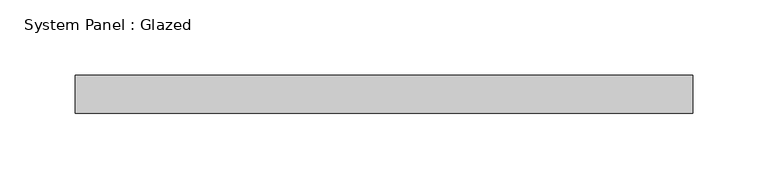
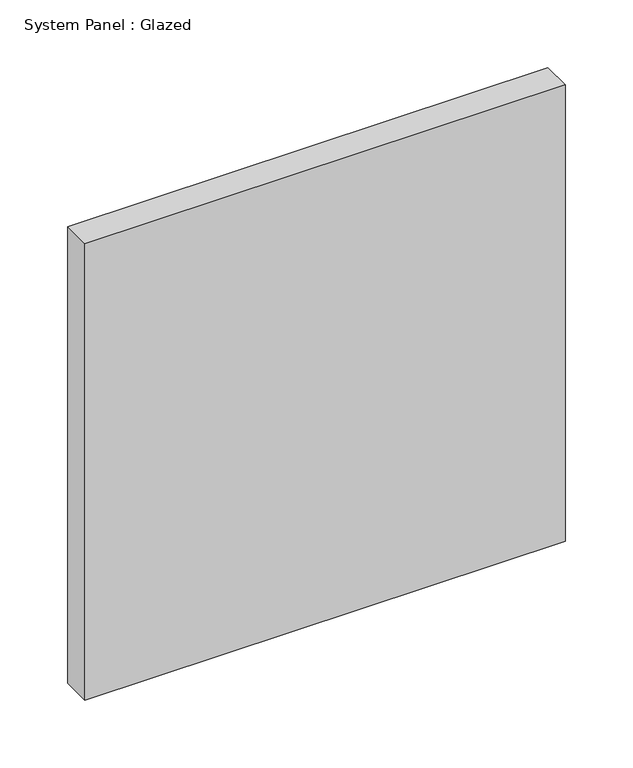
"""IFC4 building model written with IfcOpenShell, lengths in millimetres: plate geometry, System Panel : Glazed."""

from ifc_helpers import new_model, si_unit, origin, origin_with_axes, place, context, project, spatial, polyline, outline, extrude, source, transform, mapped, element, save


def system_panel_glazed_3f4378e1(model_context):
    return source(origin(), model_context, "Body", "SweptSolid", [
        extrude(outline(polyline([(205.3166667, 19.05), (-205.3166667, 19.05), (-205.3166667, 44.45), (205.3166667, 44.45), (205.3166667, 19.05)])), origin_with_axes(), (0.0, 0.0, 1.0), 412.75),
    ])


if __name__ == "__main__":
    model = new_model("IFC4")
    model_context = context("Model", 3, world=origin())
    ifc_project = project(units=[si_unit("LENGTHUNIT", "METRE", prefix="MILLI")], contexts=[model_context])
    site = spatial("IfcSite", under=ifc_project)
    building = spatial("IfcBuilding", under=site)
    placement = place(None, origin())
    system_panel_glazed_shape = system_panel_glazed_3f4378e1(model_context)
    element("IfcPlate", 1, ObjectType="System Panel : Glazed", at=placement, inside=building, context=model_context, shape_type="MappedRepresentation", body=[
        mapped(system_panel_glazed_shape, transform((0.0, 0.0, 0.0), x_axis=(1.0, 0.0, 0.0), y_axis=(0.0, 1.0, 0.0), z_axis=(0.0, 0.0, 1.0))),
    ])
    save(model, "model.ifc")

# Revit data of these elements
# Type "System Panel : Glazed"
#   Construction Type Id = "GSP4R"
#   Analytic Construction = "1/8 in Pilkington single glazing"
#   Visual Light Transmittance = 0.9
#   Solar Heat Gain Coefficient = 0.86
#   Heat Transfer Coefficient (U) = 1.18115 BTU/(h·ft²·°F)
#   Define Thermal Properties by = 1
# Element 1 (IfcPlate, "System Panel : Glazed")
#   Materials on its faces: "Glass"
# Materials
#   "Glass": class "Glass", colour RGB 0 128 192, transparency 0.75, Description = "Soda Lime Glass", Cost = 0
